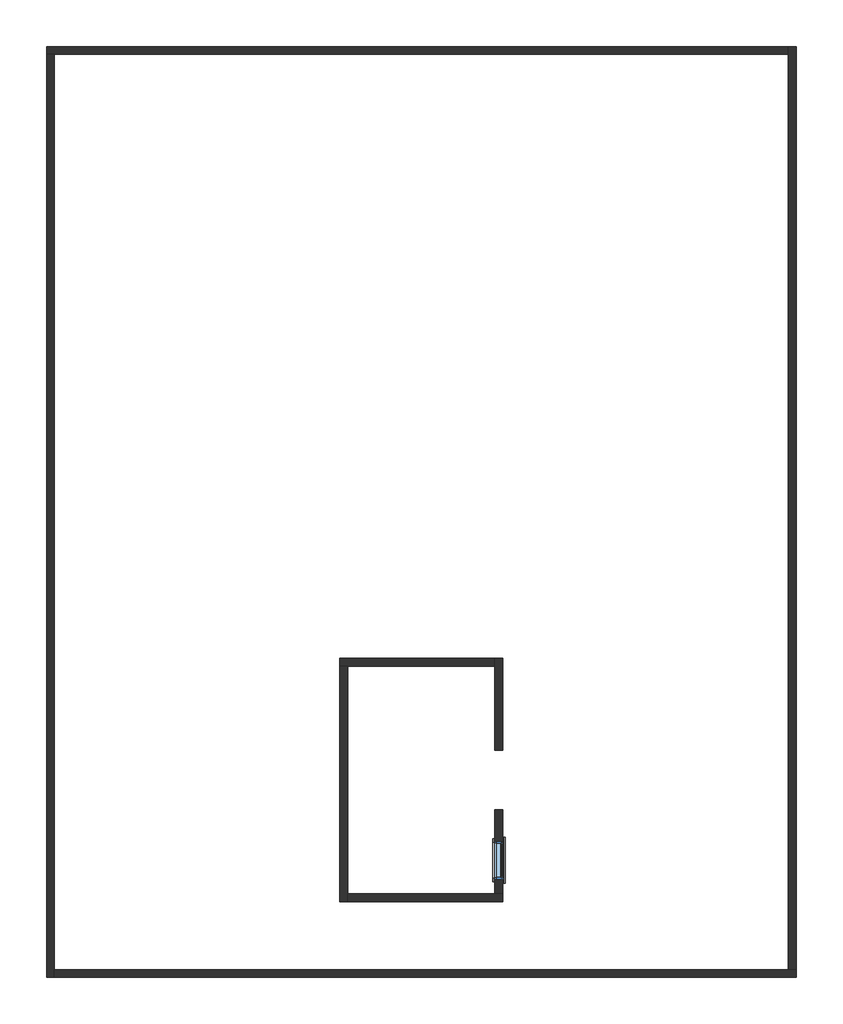
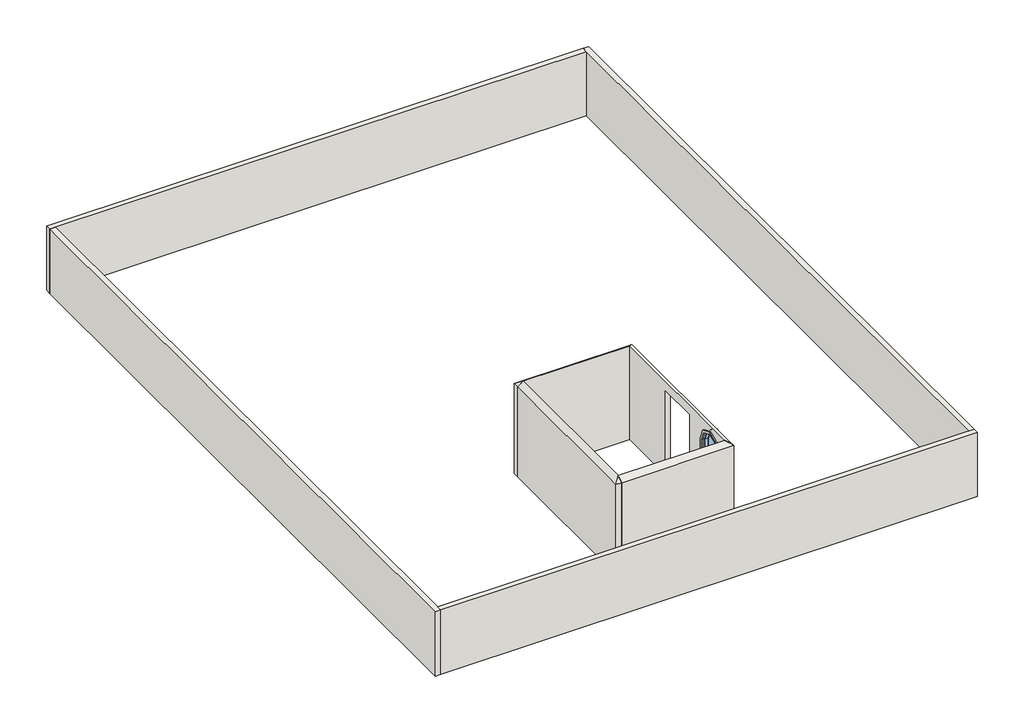
# One storey: 8 walls, 2 proxies, 1 window.
"""IFC4 building model written with IfcOpenShell, lengths in millimetres."""

from ifc_helpers import new_model, si_unit, frame, origin, place, context, project, spatial, polyline, circle_curve, faceted_brep, transform, mapped, element, save
from ifc_brep_helpers import plane_surface, revolved_surface, advanced_brep
from components import trim_window_exterior_flat_arch_top_tree_centered_with_sill_b3d54518, trim_window_interior_flat_arch_top_tree_centered_picture_1d59b3d4, window_d6aed77d

model = new_model("IFC4")

# Units and contexts
model_context = context("Model", 3, world=origin())
ifc_project = project(units=[si_unit("LENGTHUNIT", "METRE", prefix="MILLI")], contexts=[model_context])

# Site, building, storey
site = spatial("IfcSite", under=ifc_project)
building = spatial("IfcBuilding", under=site)
storey = spatial("IfcBuildingStorey", under=building, Elevation=6553.2)

# Proxies
placement = place(None, origin())
trim_window_exterior_flat_arch_top_tree_centered_with_sill_shape = trim_window_exterior_flat_arch_top_tree_centered_with_sill_b3d54518(model_context)
element("IfcBuildingElementProxy", 1, Name="Trim-Window-Exterior-Flat-Arch-Top-Tree_Centered : with Sill", ObjectType="Trim-Window-Exterior-Flat-Arch-Top-Tree_Centered : with Sill", at=placement, inside=storey, context=model_context, shape_type="MappedRepresentation", body=[
    mapped(trim_window_exterior_flat_arch_top_tree_centered_with_sill_shape, transform((-8218.1771954, -4630.7552609, 8611.0304612), x_axis=(0.0, 1.0, 0.0), y_axis=(0.0, 0.0, 1.0), z_axis=(1.0, 0.0, 0.0))),
])
trim_window_interior_flat_arch_top_tree_centered_picture_shape = trim_window_interior_flat_arch_top_tree_centered_picture_1d59b3d4(model_context)
element("IfcBuildingElementProxy", 2, Name="Trim-Window-Interior-Flat-Arch-Top-Tree_Centered : Picture Frame", ObjectType="Trim-Window-Interior-Flat-Arch-Top-Tree_Centered : Picture Frame", at=placement, inside=storey, context=model_context, shape_type="MappedRepresentation", body=[
    mapped(trim_window_interior_flat_arch_top_tree_centered_picture_shape, transform((-8345.1771954, -4630.7552609, 8611.0304612), x_axis=(0.0, -1.0, 0.0), y_axis=(0.0, 0.0, 1.0), z_axis=(-1.0, 0.0, 0.0))),
])

# Walls
element("IfcWall", 3, ObjectType="INNER WALL 5\"", at=placement, inside=storey, context=model_context, shape_type="Brep", body=[
    faceted_brep([(-10859.7771954, -1477.6727897, 6553.2), (-10732.7771954, -1477.6727897, 6553.2), (-8345.1771954, -1477.6727897, 6553.2), (-8345.1771954, -1477.6727897, 8782.05), (-10732.7771954, -1477.6727897, 8782.05), (-10859.7771954, -1477.6727897, 8686.8), (-10859.7771954, -1350.6727897, 6553.2), (-10859.7771954, -1350.6727897, 8686.8), (-8345.1771954, -1350.6727897, 8686.8), (-8345.1771954, -1350.6727897, 6553.2)], [[[0, 1, 2, 3, 4, 5]], [[6, 7, 8, 9]], [[2, 1, 0, 6, 9]], [[0, 5, 7, 6]], [[3, 2, 9, 8]], [[5, 4, 7]], [[4, 3, 8, 7]]]),
])
element("IfcWall", 4, ObjectType="INNER WALL 5\"", at=placement, inside=storey, context=model_context, shape_type="Brep", body=[
    faceted_brep([(-10732.7771954, -5303.8552609, 6553.2), (-10732.7771954, -5176.8552609, 6553.2), (-10732.7771954, -1477.6727897, 6553.2), (-10732.7771954, -1477.6727897, 8782.05), (-10732.7771954, -5176.8552609, 8782.05), (-10732.7771954, -5303.8552609, 8686.8), (-10859.7771954, -5303.8552609, 6553.2), (-10859.7771954, -5303.8552609, 8686.8), (-10859.7771954, -1477.6727897, 8686.8), (-10859.7771954, -1477.6727897, 6553.2)], [[[0, 1, 2, 3, 4, 5]], [[6, 7, 8, 9]], [[2, 1, 0, 6, 9]], [[0, 5, 7, 6]], [[3, 2, 9, 8]], [[5, 4, 7]], [[4, 3, 8, 7]]]),
])
element("IfcWall", 5, ObjectType="INNER WALL 5\"", at=placement, inside=storey, context=model_context, shape_type="Brep", body=[
    faceted_brep([(-8218.1771954, -5176.8552609, 6553.2), (-8345.1771954, -5176.8552609, 6553.2), (-10732.7771954, -5176.8552609, 6553.2), (-10732.7771954, -5176.8552609, 8782.05), (-8345.1771954, -5176.8552609, 8782.05), (-8218.1771954, -5176.8552609, 8686.8), (-8218.1771954, -5303.8552609, 6553.2), (-8218.1771954, -5303.8552609, 8686.8), (-10732.7771954, -5303.8552609, 8686.8), (-10732.7771954, -5303.8552609, 6553.2)], [[[0, 1, 2, 3, 4, 5]], [[6, 7, 8, 9]], [[2, 1, 0, 6, 9]], [[0, 5, 7, 6]], [[3, 2, 9, 8]], [[5, 4, 7]], [[4, 3, 8, 7]]]),
])
element("IfcWall", 6, ObjectType="INNER WALL 5\"", at=placement, inside=storey, context=model_context, shape_type="AdvancedBrep", body=[
    advanced_brep(
    [(-8345.1771954, -1350.6727897, 8686.8), (-8345.1771954, -1350.6727897, 6553.2), (-8345.1771954, -1477.6727897, 6553.2), (-8345.1771954, -2844.6640253, 6553.2), (-8345.1771954, -2844.6640253, 8559.8), (-8345.1771954, -3809.8640253, 8559.8), (-8345.1771954, -3809.8640253, 6553.2), (-8345.1771954, -5176.8552609, 6553.2), (-8345.1771954, -5176.8552609, 8782.05), (-8345.1771954, -1477.6727897, 8782.05), (-8345.1771954, -4325.9552609, 7696.6304612), (-8345.1771954, -4325.9552609, 8306.2304612), (-8345.1771954, -4935.5552609, 8306.2304612), (-8345.1771954, -4935.5552609, 7696.6304612), (-8218.1771954, -1350.6727897, 8686.8), (-8218.1771954, -5176.8552609, 8686.8), (-8218.1771954, -5176.8552609, 6553.2), (-8218.1771954, -3809.8640253, 6553.2), (-8218.1771954, -3809.8640253, 8559.8), (-8218.1771954, -2844.6640253, 8559.8), (-8218.1771954, -2844.6640253, 6553.2), (-8218.1771954, -1350.6727897, 6553.2), (-8218.1771954, -4325.9552609, 7696.6304612), (-8218.1771954, -4935.5552609, 7696.6304612), (-8218.1771954, -4935.5552609, 8306.2304612), (-8218.1771954, -4325.9552609, 8306.2304612)],
    [
        (0, 1),
        (1, 2),
        (2, 3),
        (3, 4),
        (4, 5),
        (5, 6),
        (6, 7),
        (7, 8),
        (8, 9),
        (9, 0),
        (10, 11),
        (11, 12, circle_curve(frame((-8345.1771954, -4630.7552609, 8306.2304612), z_axis=(1.0, 0.0, 0.0), x_axis=(0.0, -1.0, 0.0)), 304.8)),
        (12, 13),
        (13, 10),
        (14, 15),
        (15, 16),
        (16, 17),
        (17, 18),
        (18, 19),
        (19, 20),
        (20, 21),
        (21, 14),
        (22, 23),
        (23, 24),
        (24, 25, circle_curve(frame((-8218.1771954, -4630.7552609, 8306.2304612), z_axis=(-1.0, 0.0, 0.0), x_axis=(0.0, -1.0, 0.0)), 304.8)),
        (25, 22),
        (1, 21),
        (20, 3),
        (16, 7),
        (6, 17),
        (0, 14),
        (15, 8),
        (5, 18),
        (4, 19),
        (22, 10),
        (13, 23),
        (12, 24),
        (11, 25),
        (9, 14),
    ],
    [
        plane_surface(frame((-8345.1771954, -1414.1727897, 6553.2), z_axis=(-1.0, 0.0, 0.0), x_axis=(0.0, -1.0, 0.0))),
        plane_surface(frame((-8218.1771954, -1414.1727897, 6553.2), z_axis=(1.0, 0.0, 0.0), x_axis=(0.0, 1.0, 0.0))),
        plane_surface(frame((-8345.1771954, -1414.1727897, 6553.2), z_axis=(0.0, 0.0, -1.0), x_axis=(1.0, 0.0, 0.0))),
        plane_surface(frame((-10796.2771954, -1350.6727897, 6553.2), z_axis=(0.0, 1.0, 0.0), x_axis=(-1.0, 0.0, 0.0))),
        plane_surface(frame((-8281.6771954, -5176.8552609, 6553.2), z_axis=(0.0, -1.0, 0.0), x_axis=(-1.0, 0.0, 0.0))),
        plane_surface(frame((-9869.1771954, -3809.8640253, 6400.8), z_axis=(0.0, 1.0, 0.0), x_axis=(1.0, 0.0, 0.0))),
        plane_surface(frame((-9869.1771954, -3809.8640253, 8559.8), z_axis=(0.0, 0.0, -1.0), x_axis=(1.0, 0.0, 0.0))),
        plane_surface(frame((-9869.1771954, -2844.6640253, 8559.8), z_axis=(0.0, -1.0, 0.0), x_axis=(1.0, 0.0, 0.0))),
        plane_surface(frame((-8218.1771954, -4325.9552609, 7696.6304612), z_axis=(0.0, 0.0, 1.0), x_axis=(-1.0, 0.0, 0.0))),
        plane_surface(frame((-8218.1771954, -4935.5552609, 7696.6304612), z_axis=(0.0, 1.0, 0.0), x_axis=(-1.0, 0.0, 0.0))),
        revolved_surface(polyline([(-8345.1771954, -4935.555260900001, 8306.2304612), (-8218.1771954, -4935.555260900001, 8306.2304612)]), (-8345.1771954, -4630.7552609, 8306.2304612), (-1.0, 0.0, 0.0)),
        plane_surface(frame((-8218.1771954, -4325.9552609, 8306.2304612), z_axis=(0.0, -1.0, 0.0), x_axis=(-1.0, 0.0, 0.0))),
        plane_surface(frame((-8218.1771954, -1350.6727897, 8686.8), z_axis=(0.0, 0.6, 0.8), x_axis=(-1.0, 0.0, 0.0))),
        plane_surface(frame((-8218.1771954, -5303.8552609, 8686.8), z_axis=(0.5999999999999996, 0.0, 0.8000000000000004), x_axis=(0.0, 1.0, 0.0))),
    ],
    [
        (0, [[1, 2, 3, 4, 5, 6, 7, 8, 9, 10], [11, 12, 13, 14]]),
        (1, [[15, 16, 17, 18, 19, 20, 21, 22], [23, 24, 25, 26]]),
        (2, [[27, -21, 28, -3, -2]]),
        (2, [[29, -7, 30, -17]]),
        (3, [[-1, 31, -22, -27]]),
        (4, [[-8, -29, -16, 32]]),
        (5, [[33, -18, -30, -6]]),
        (6, [[-33, -5, 34, -19]]),
        (7, [[-34, -4, -28, -20]]),
        (8, [[-23, 35, -14, 36]]),
        (9, [[-24, -36, -13, 37]]),
        (10, [[-25, -37, -12, 38]]),
        (11, [[-26, -38, -11, -35]]),
        (12, [[-31, -10, 39]]),
        (13, [[-15, -39, -9, -32]]),
    ],
),
])
element("IfcWall", 7, ObjectType="INNER WALL 5\"", at=placement, inside=storey, context=model_context, shape_type="Brep", body=[
    faceted_brep([(-3455.6771954, -6405.2727897, 6553.2), (-3582.6771954, -6405.2727897, 6553.2), (-15496.8646954, -6405.2727897, 6553.2), (-15496.8646954, -6405.2727897, 8077.2), (-3582.6771954, -6405.2727897, 8077.2), (-3455.6771954, -6405.2727897, 8077.2), (-3455.6771954, -6532.2727897, 6553.2), (-3455.6771954, -6532.2727897, 8077.2), (-15496.8646954, -6532.2727897, 8077.2), (-15496.8646954, -6532.2727897, 6553.2)], [[[0, 1, 2, 3, 4, 5]], [[6, 7, 8, 9]], [[2, 1, 0, 6, 9]], [[5, 4, 3, 8, 7]], [[0, 5, 7, 6]], [[3, 2, 9, 8]]]),
])
element("IfcWall", 8, ObjectType="INNER WALL 5\"", at=placement, inside=storey, context=model_context, shape_type="Brep", body=[
    faceted_brep([(-3582.6771954, 8580.7272103, 6553.2), (-3582.6771954, 8453.7272103, 6553.2), (-3582.6771954, -6405.2727897, 6553.2), (-3582.6771954, -6405.2727897, 8077.2), (-3582.6771954, 8453.7272103, 8077.2), (-3582.6771954, 8580.7272103, 8077.2), (-3455.6771954, 8580.7272103, 6553.2), (-3455.6771954, 8580.7272103, 8077.2), (-3455.6771954, -6405.2727897, 8077.2), (-3455.6771954, -6405.2727897, 6553.2)], [[[0, 1, 2, 3, 4, 5]], [[6, 7, 8, 9]], [[2, 1, 0, 6, 9]], [[5, 4, 3, 8, 7]], [[0, 5, 7, 6]], [[3, 2, 9, 8]]]),
])
element("IfcWall", 9, ObjectType="INNER WALL 5\"", at=placement, inside=storey, context=model_context, shape_type="Brep", body=[
    faceted_brep([(-15623.8646954, 8453.7272103, 6553.2), (-15496.8646954, 8453.7272103, 6553.2), (-3582.6771954, 8453.7272103, 6553.2), (-3582.6771954, 8453.7272103, 8077.2), (-15496.8646954, 8453.7272103, 8077.2), (-15623.8646954, 8453.7272103, 8077.2), (-15623.8646954, 8580.7272103, 6553.2), (-15623.8646954, 8580.7272103, 8077.2), (-3582.6771954, 8580.7272103, 8077.2), (-3582.6771954, 8580.7272103, 6553.2)], [[[0, 1, 2, 3, 4, 5]], [[6, 7, 8, 9]], [[2, 1, 0, 6, 9]], [[5, 4, 3, 8, 7]], [[0, 5, 7, 6]], [[3, 2, 9, 8]]]),
])
element("IfcWall", 10, ObjectType="INNER WALL 5\"", at=placement, inside=storey, context=model_context, shape_type="Brep", body=[
    faceted_brep([(-15496.8646954, -6532.2727897, 6553.2), (-15496.8646954, -6405.2727897, 6553.2), (-15496.8646954, 8453.7272103, 6553.2), (-15496.8646954, 8453.7272103, 8077.2), (-15496.8646954, -6405.2727897, 8077.2), (-15496.8646954, -6532.2727897, 8077.2), (-15623.8646954, -6532.2727897, 6553.2), (-15623.8646954, -6532.2727897, 8077.2), (-15623.8646954, 8453.7272103, 8077.2), (-15623.8646954, 8453.7272103, 6553.2)], [[[0, 1, 2, 3, 4, 5]], [[6, 7, 8, 9]], [[2, 1, 0, 6, 9]], [[5, 4, 3, 8, 7]], [[0, 5, 7, 6]], [[3, 2, 9, 8]]]),
])

# Window
window_shape = window_d6aed77d(model_context)
element("IfcWindow", 11, ObjectType="Window-Fixed-Round-Top : 24\" x 36\"", at=placement, inside=storey, context=model_context, shape_type="MappedRepresentation", body=[
    mapped(window_shape, transform((-8281.6771954, -4630.7552609, 6782.2304612), x_axis=(0.0, -1.0, 0.0), y_axis=(1.0, 0.0, 0.0), z_axis=(0.0, 0.0, 1.0))),
])

save(model, "model.ifc")

# Revit data of these elements
# Type "Trim-Window-Exterior-Flat-Arch-Top-Tree_Centered : with Sill"
#   Trim Width = 0' - 2 1/4"
#   Trim Thickness_Picture Frame = 0' - 1 1/4"
#   Trim Thickness_with Sill = 0' - 0 3/4"
#   Sill Thickness = 0' - 1 1/4"
#   Opening Width [instance default] = 2' - 0"
#   Opening Height [instance default] = 3' - 0"
#   Default Elevation = 4' - 0"
#   Sill = yes
#   Picture Frame = no
#   Trim Material [instance default] = none
# Type "Trim-Window-Interior-Flat-Arch-Top-Tree_Centered : Picture Frame"
#   Trim Thickness_Picture Frame = 0' - 1 1/4"
#   Trim Width = 0' - 2 1/4"
#   Trim Thickness_with Sill = 0' - 0 3/4"
#   Sill Thickness = 0' - 1 1/4"
#   Opening Width [instance default] = 2' - 0"
#   Opening Height [instance default] = 3' - 0"
#   Default Elevation = 4' - 0"
#   Sill = no
#   Picture Frame = yes
#   Trim Material [instance default] = none
# Type "INNER WALL 5\""
#   Assembly Code = "B2010"
#   Layers, outside or top first: 0' - 5" "OUTER WALL PAINT" (function 1)
# Type "Window-Fixed-Round-Top : 24\" x 36\""
#   Type Mark = "31"
#   Fire Rating = "0.5h"
#   Assembly Code = "B2020100"
#   Analytic Construction = "Double glazing - domestic"
#   Window Inset [instance default] = 0' - 0"
#   Wall Thickness [instance default] = 0' - 6"
#   Visual Light Transmittance = 0.81
#   Thermal Resistance (R) = 1.8146 (h·ft²·°F)/BTU
#   Solar Heat Gain Coefficient = 0.76
#   Rough Width = 2' - 0 1/2"
#   Rough Height = 3' - 0 1/2"
#   Interior Wall Closure [instance default] = 0' - 2 1/4"
#   Height = 3' - 0"
#   Heat Transfer Coefficient (U) = 0.5511 BTU/(h·ft²·°F)
#   Frame Extension [instance default] = 0' - 0 1/4"
#   Exterior Wall Closure [instance default] = 0' - 1 1/4"
#   Extension Jamb [instance default] = 0' - 2 1/4"
#   Default Sill Height = 3' - 0"
#   Width = 2' - 0"
#   Interior Trim Visibility [instance default] = yes
#   Exterior Trim Visibility [instance default] = yes
#   Extension Jamb Visibility [instance default] = yes
#   Interior Trim Material = Wood - Stained
#   Interior Trim = Trim-Window-Interior-Flat-Arch-Top-Tree_Centered : Picture Frame
#   Interior Frame Material = Wood - Stained
#   Glass Panel Material = Glass
#   Exterior Trim Material = Clad - White
#   Exterior Trim = Trim-Window-Exterior-Flat-Arch-Top-Tree_Centered : with Sill
#   Exterior Frame Material = Clad - White
#   Wall Closure = (empty or 0)
# Element 1 (IfcBuildingElementProxy, "Trim-Window-Exterior-Flat-Arch-Top-Tree_Centered : with Sill")
#   Opening Width = 2' - 0"
#   Opening Height = 3' - 0"
#   Trim Material = Clad - White
#   Phase Created = New Construction
#   Materials on its faces: "Clad - White"
# Element 2 (IfcBuildingElementProxy, "Trim-Window-Interior-Flat-Arch-Top-Tree_Centered : Picture Frame")
#   Opening Width = 2' - 0"
#   Opening Height = 3' - 0"
#   Trim Material = Wood - Stained
#   Phase Created = New Construction
#   Materials on its faces: "Wood - Stained"
# Elements 3, 4, 6 (IfcWall, "INNER WALL 5\"")
#   Top Offset = 0' - 0"
#   Base Offset = 0' - 0"
#   Unconnected Height = 7' - 0"
#   wall height = 7' - 0"
#   Phase Created = New Construction
#   Base Constraint = SLB 6
#   Materials on its faces: "OUTER WALL PAINT"
# Element 5 (IfcWall, "INNER WALL 5\"")
#   Top Offset = 0' - 0"
#   Base Offset = 0' - 0"
#   Unconnected Height = 7' - 0"
#   wall height = 7' - 0"
#   Phase Created = New Construction
#   Base Constraint = SLB 6
#   Materials on its faces: "OUTER WALL PAINT", "Porcelain, Ivory"
# Elements 7, 8, 9, 10 (IfcWall, "INNER WALL 5\"")
#   Top Offset = 0' - 0"
#   Base Offset = 0' - 0"
#   Unconnected Height = 5' - 0"
#   wall height = 5' - 0"
#   Phase Created = New Construction
#   Base Constraint = SLB 6
#   Materials on its faces: "OUTER WALL PAINT", "outer wall paint 234"
# Element 11 (IfcWindow, "Window-Fixed-Round-Top : 24\" x 36\"")
#   Mark = "47"
#   Window Inset = 0' - 0"
#   Interior Wall Closure = 0' - 2 1/4"
#   Frame Extension = 0' - 0 1/4"
#   Exterior Wall Closure = 0' - 1 1/4"
#   Interior Trim Visibility = yes
#   Exterior Trim Visibility = yes
#   Phase Created = New Construction
#   Materials on its faces: "Wood - Stained", "Clad - White", "Glass"
# Materials
#   "OUTER WALL PAINT": class "Generic", colour RGB 120 120 120, transparency 0, Cost = 0
#   "Wood - Stained": class "Wood", colour RGB 224 178 126, transparency 0, Cost = 0
#   "Glass": class "Glass", colour RGB 0 128 192, transparency 0.75, Description = "Soda Lime Glass", Cost = 0
#   "Clad - White": class "Wood", colour RGB 242 242 238, transparency 0, Cost = 0
#   "Porcelain, Ivory": class "Ceramic", colour RGB 247 247 239, transparency 0, Description = "Porcelain, ivory", Cost = 0
#   "outer wall paint 234": class "Generic", colour RGB 120 120 120, transparency 0, Cost = 0
